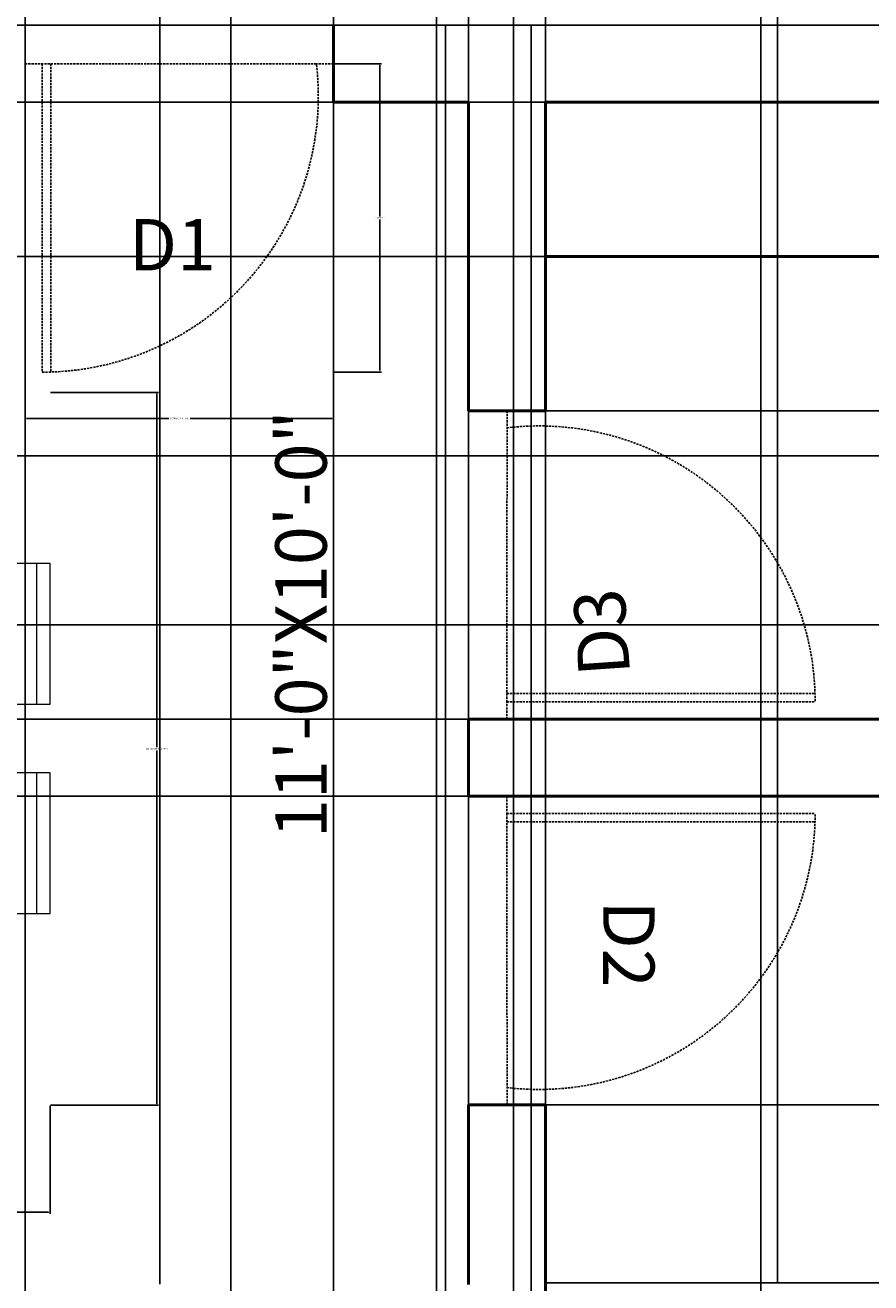
# Model space of a CAD drawing. Units: inches. Extents: x 3 to 576, y -689 to 51.
# Tile 10 of 21: x 336 to 435, y -506 to -359. Entities that reach past the tile are written whole.
import ezdxf

# ---------------------------------------------------------------- set-up
doc = ezdxf.new("R2010")
doc.units = ezdxf.units.IN
doc.header["$MEASUREMENT"] = 0
doc.linetypes.add('DASHED2', pattern=[0.375, 0.25, -0.125])
for name, color, linetype, lineweight in [('A-ANNO-DIMS', 2, 'Continuous', 18), ('A-ANNO-TEXT', 3, 'Continuous', 18), ('A-AREA-IDEN', 7, 'Continuous', 18), ('A-DOOR', 4, 'DASHED2', 25), ('A-FURN', 8, 'Continuous', 18), ('A-WALL', 7, 'Continuous', 50)]:
    doc.layers.add(name, color=color, linetype=linetype, lineweight=lineweight)
doc.styles.get("Standard").update_dxf_attribs({"font": 'arial.ttf'})
doc.dimstyles.get("Standard").update_dxf_attribs({"dimtxt": 0.18, "dimasz": 0.18, "dimexe": 0.18, "dimexo": 0.0625, "dimgap": 0.09, "dimtad": 0, "dimtih": 1, "dimtoh": 1, "dimdec": 0, "dimzin": 0, "dimdsep": 46, "dimlunit": 3, "dimtxsty": 'Standard', "dimcen": 0.09, "dimadec": 0, "dimazin": 0, "dimtfac": 1, "dimtdec": 0, "dimtofl": 0, "dimtmove": 0, "dimatfit": 3, "dimfxl": 1, "dimtolj": 1, "dimtzin": 0, "dimarcsym": 0})

# ---------------------------------------------------------------- blocks, each defined once
blk = doc.blocks.new('DINING-SET-6')
for p, q in [((35.44, 83.21), (19.03, 83.21)), ((19.03, 83.21), (19.03, 74.43)), ((35.44, 74.43), (35.44, 83.21)), ((19.03, 81.61), (35.44, 81.61)), ((37.96, 74.43), (16.08, 74.43)), ((16.08, 72.6), (37.96, 72.6)), ((8.79, 67.13), (8.79, 16.08)), ((10.61, 16.08), (10.61, 67.13)), ((20.49, 66.46), (21.48, 64.87)), ((43.43, 67.13), (43.43, 16.08)), ((45.25, 16.08), (45.25, 67.13)), ((21.9, 63.9), (21.31, 65.43)), ((22.64, 64.98), (21.31, 65.43)), ((21.48, 64.87), (23.07, 63.29)), ((21.9, 63.9), (22.63, 64.98)), ((0, 46.82), (0, 63.23)), ((0, 63.23), (8.79, 63.23)), ((1.6, 63.23), (1.6, 46.82)), ((12.38, 64.08), (12.77, 63.09)), ((23.07, 63.29), (24.85, 62.49)), ((54.04, 63.23), (45.25, 63.23)), ((52.44, 63.23), (52.44, 46.82)), ((54.04, 46.82), (54.04, 63.23)), ((12.77, 63.09), (14.75, 59.12)), ((24.85, 62.49), (25.84, 62.3)), ((25.84, 62.3), (26.44, 61.7)), ((26.44, 61.7), (27.43, 60.91)), ((29.06, 62.49), (27.69, 62.24)), ((28.94, 61.18), (27.69, 62.24)), ((28.94, 61.18), (29.06, 62.49)), ((27.43, 60.91), (28.22, 59.52)), ((12.6, 59.46), (11.23, 59.2)), ((12.49, 58.15), (11.23, 59.2)), ((12.49, 58.15), (12.6, 59.46)), ((14.75, 59.12), (17.52, 55.75)), ((28.22, 59.52), (29.6, 56.55)), ((38.5, 59.66), (37.18, 60.1)), ((37.77, 58.57), (37.18, 60.1)), ((37.77, 58.57), (38.5, 59.66)), ((26.06, 56.77), (23.98, 56.52)), ((25.76, 54.82), (23.98, 56.52)), ((25.76, 54.82), (26.06, 56.77)), ((29.6, 56.55), (30.2, 54.36)), ((30, 56.15), (30.79, 55.36)), ((17.52, 55.75), (18.51, 53.57)), ((30.2, 54.36), (31.39, 52.78)), ((30.79, 55.36), (32.18, 53.97)), ((18.51, 53.57), (18.51, 49.01)), ((32.18, 53.97), (33.96, 53.37)), ((33.96, 53.37), (34.36, 53.18)), ((34.36, 53.18), (35.35, 49.61)), ((13.09, 50.84), (12.5, 52.37)), ((13.83, 51.93), (12.5, 52.37)), ((13.09, 50.84), (13.83, 51.92)), ((31.39, 52.78), (32.77, 51.19)), ((19.11, 51.19), (19.11, 50)), ((19.11, 50), (19.5, 47.82)), ((32.77, 51.19), (33.76, 50.4)), ((33.76, 50.4), (34.75, 46.83)), ((41.09, 49.61), (41.49, 50)), ((18.51, 49.01), (17.52, 46.63)), ((35.35, 49.61), (36.73, 48.22)), ((39.5, 47.23), (41.09, 49.61)), ((43.43, 49.7), (42.77, 49.58)), ((43.43, 49.03), (42.77, 49.58)), ((19.5, 47.82), (19.5, 36.32)), ((28.96, 45.51), (28.37, 47.05)), ((29.69, 46.6), (28.37, 47.05)), ((36.73, 48.22), (37.92, 47.62)), ((37.92, 47.62), (38.71, 47.62)), ((38.71, 47.62), (39.5, 47.23)), ((8.79, 46.82), (0, 46.82)), ((17.52, 46.63), (17.92, 44.25)), ((27.69, 46.8), (26.31, 46.55)), ((27.57, 45.49), (26.31, 46.55)), ((27.57, 45.49), (27.68, 46.8)), ((28.96, 45.51), (29.69, 46.6)), ((34.75, 46.83), (35.15, 44.25)), ((45.25, 46.82), (54.04, 46.82)), ((17.92, 44.25), (18.12, 43.46)), ((19.5, 44.06), (20.09, 43.66)), ((35.15, 44.25), (35.54, 43.06)), ((11.23, 43.76), (10.61, 43.65)), ((11.11, 42.46), (10.61, 42.88)), ((11.11, 42.46), (11.23, 43.76)), ((20.09, 43.66), (21.08, 43.07)), ((21.08, 43.07), (21.68, 42.27)), ((35.54, 43.06), (35.15, 41.68)), ((21.68, 42.27), (22.67, 41.88)), ((22.67, 41.88), (23.46, 41.68)), ((23.46, 41.68), (23.85, 41.68)), ((23.85, 41.68), (24.45, 41.48)), ((35.15, 41.68), (36.14, 40.29)), ((36.14, 40.29), (36.73, 37.12)), ((0, 22.39), (0, 38.8)), ((0, 38.8), (8.79, 38.8)), ((1.6, 38.8), (1.6, 22.39)), ((54.04, 38.8), (45.25, 38.8)), ((52.44, 38.8), (52.44, 22.39)), ((54.04, 22.39), (54.04, 38.8)), ((19.5, 36.32), (19.9, 35.93)), ((19.9, 35.93), (23.27, 33.35)), ((20.15, 32.45), (19.56, 33.99)), ((20.88, 33.54), (19.56, 33.99)), ((42.77, 34.14), (41.4, 33.89)), ((42.65, 32.83), (41.4, 33.89)), ((42.65, 32.83), (42.77, 34.14)), ((20.15, 32.45), (20.88, 33.54)), ((22.44, 33.42), (20.36, 33.17)), ((22.14, 31.47), (20.36, 33.17)), ((22.14, 31.47), (22.44, 33.42)), ((23.27, 33.35), (26.24, 31.57)), ((23.86, 32.95), (25.64, 32.95)), ((25.64, 32.95), (27.03, 32.16)), ((26.31, 31.11), (24.94, 30.85)), ((26.2, 29.8), (24.94, 30.85)), ((26.24, 31.57), (25.84, 28.59)), ((26.2, 29.8), (26.31, 31.11)), ((27.03, 32.16), (27.82, 31.37)), ((27.82, 31.37), (28.81, 30.57)), ((25.84, 28.59), (25.84, 28)), ((36.01, 27.13), (35.43, 28.66)), ((36.75, 28.22), (35.43, 28.66)), ((36.01, 27.13), (36.75, 28.22)), ((40.69, 28), (38.9, 24.23)), ((38.9, 24.23), (38.9, 23.44)), ((8.79, 22.39), (0, 22.39)), ((38.9, 23.44), (39.3, 22.45)), ((39.3, 22.45), (38.9, 20.86)), ((45.25, 22.39), (54.04, 22.39)), ((11.34, 19.39), (10.75, 20.93)), ((12.07, 20.48), (10.75, 20.93)), ((38.9, 20.86), (37.72, 19.87)), ((11.34, 19.39), (12.07, 20.48)), ((30.99, 19.67), (29.8, 20.27)), ((31.78, 16.89), (30.99, 19.67)), ((37.72, 19.87), (37.52, 18.09)), ((37.52, 18.09), (36.92, 16.1)), ((41.28, 17.14), (40.02, 18.2)), ((41.4, 18.45), (40.03, 18.2)), ((41.28, 17.14), (41.4, 18.45)), ((32.18, 16.5), (31.78, 16.89)), ((32.57, 12.93), (32.18, 16.5)), ((24.94, 15.41), (23.57, 15.16)), ((24.82, 14.11), (23.57, 15.16)), ((24.82, 14.11), (24.94, 15.41)), ((27.21, 14.07), (26.62, 15.6)), ((27.94, 15.16), (26.62, 15.6)), ((27.21, 14.07), (27.94, 15.16)), ((36.13, 15.11), (35.74, 14.52)), ((36.92, 16.1), (36.13, 15.11)), ((32.57, 12.53), (32.57, 12.93)), ((35.15, 11.94), (32.57, 12.53)), ((36.14, 11.15), (35.15, 11.94)), ((42.34, 12.8), (41.67, 12.72)), ((42.01, 12.4), (41.67, 12.72)), ((37.96, 10.61), (16.08, 10.61)), ((37.13, 10.75), (36.14, 11.15)), ((16.08, 8.79), (37.96, 8.79)), ((19.03, 8.79), (19.03, 0)), ((35.44, 0), (35.44, 8.79)), ((35.44, 1.6), (19.03, 1.6)), ((19.03, 0), (35.44, 0))]:
    blk.add_line(p, q)
for centre, radius, start, end in [((16.08, 67.13), 7.29, 90, 180), ((37.96, 67.13), 7.29, 0, 90), ((16.08, 67.13), 5.47, 90, 180), ((37.96, 67.13), 5.47, 0, 90), ((16.08, 16.08), 7.29, 180, 270), ((16.08, 16.08), 5.47, 180, 270), ((37.96, 16.08), 5.47, 270, 0), ((37.96, 16.08), 7.29, 270, 0)]:
    blk.add_arc(centre, radius, start, end)
blk = doc.blocks.new('DOOR-SWING-900')
for p, q in [((35.95, 36), (35.95, 34)), ((36, 2), (35.95, 34)), ((36, 2), (0, 2)), ((36, 0), (36, 2))]:
    blk.add_line(p, q)
blk.add_arc((32.22, 2), 32.22, 83.347, 180)
blk = doc.blocks.new('DOOR-900')
for p, q in [((34, 36), (0, 36)), ((2, 36), (2, 0)), ((36, 36), (34, 36))]:
    blk.add_line(p, q)
blk.add_arc((2, 32.22), 32.22, 270, 6.7329)
blk = doc.blocks.new('*D21')
at = {"layer": 'A-ANNO-DIMS', "color": 0, "lineweight": -2, "transparency": 16777216}
for p, q in [((336.29, -399.87), (336.29, -405.39)), ((372.29, -399.87), (372.29, -405.39)), ((336.47, -405.21), (353.05, -405.21)), ((372.11, -405.21), (355.54, -405.21))]:
    blk.add_line(p, q, dxfattribs=at)
at = {"layer": 'A-ANNO-DIMS', "color": 0, "transparency": 16777216}
for points in [[(336.47, -405.18), (336.47, -405.24), (336.29, -405.21)], [(372.11, -405.18), (372.11, -405.24), (372.29, -405.21)]]:
    blk.add_solid(points, dxfattribs=at)
at = {"layer": 'Defpoints', "color": 0, "transparency": 16777216}
for p in [(336.29, -399.81), (372.29, -399.81), (372.29, -405.21)]:
    blk.add_point(p, dxfattribs=at)
at = {"layer": 'A-ANNO-DIMS', "color": 0, "transparency": 16777216, "insert": (354.29, -405.21), "char_height": 0.18, "attachment_point": 5}
blk.add_mtext('\\A1;DOOR D1 3\'-0" TYP.', dxfattribs=at)
blk = doc.blocks.new('*D22')
at = {"layer": 'A-ANNO-DIMS', "color": 0, "lineweight": -2, "transparency": 16777216}
for p, q in [((372.36, -363.81), (377.87, -363.81)), ((377.69, -363.99), (377.69, -381.63)), ((377.69, -399.63), (377.69, -381.99)), ((372.36, -399.81), (377.87, -399.81))]:
    blk.add_line(p, q, dxfattribs=at)
at = {"layer": 'A-ANNO-DIMS', "color": 0, "transparency": 16777216}
for points in [[(377.66, -363.99), (377.72, -363.99), (377.69, -363.81)], [(377.66, -399.63), (377.72, -399.63), (377.69, -399.81)]]:
    blk.add_solid(points, dxfattribs=at)
at = {"layer": 'Defpoints', "color": 0, "transparency": 16777216}
for p in [(372.29, -363.81), (377.69, -363.81), (372.29, -399.81)]:
    blk.add_point(p, dxfattribs=at)
at = {"layer": 'A-ANNO-DIMS', "color": 0, "transparency": 16777216, "insert": (377.69, -381.81), "char_height": 0.18, "attachment_point": 5}
blk.add_mtext('\\A1;3\'-0" TYP.', dxfattribs=at)
blk = doc.blocks.new('*D33')
at = {"layer": 'A-ANNO-DIMS', "color": 0, "lineweight": -2, "transparency": 16777216}
for p, q in [((339.26, -402.17), (351.86, -402.17)), ((351.68, -402.35), (351.68, -443.59)), ((351.68, -485.2), (351.68, -443.96)), ((339.26, -485.38), (351.86, -485.38))]:
    blk.add_line(p, q, dxfattribs=at)
at = {"layer": 'A-ANNO-DIMS', "color": 0, "transparency": 16777216}
for points in [[(351.65, -402.35), (351.71, -402.35), (351.68, -402.17)], [(351.65, -485.2), (351.71, -485.2), (351.68, -485.38)]]:
    blk.add_solid(points, dxfattribs=at)
at = {"layer": 'Defpoints', "color": 0, "transparency": 16777216}
for p in [(339.2, -402.17), (351.68, -402.17), (339.2, -485.38)]:
    blk.add_point(p, dxfattribs=at)
at = {"layer": 'A-ANNO-DIMS', "color": 0, "transparency": 16777216, "insert": (351.68, -443.78), "char_height": 0.18, "attachment_point": 5}
blk.add_mtext('\\A1;DINING SET 6\'-11" TYP.', dxfattribs=at)
blk = doc.blocks.new('*D34')
at = {"layer": 'A-ANNO-DIMS', "color": 0, "lineweight": -2, "transparency": 16777216}
for p, q in [((285.16, -485.45), (285.16, -498.05)), ((339.2, -485.45), (339.2, -498.05)), ((285.34, -497.87), (311.54, -497.87)), ((339.02, -497.87), (312.82, -497.87))]:
    blk.add_line(p, q, dxfattribs=at)
at = {"layer": 'A-ANNO-DIMS', "color": 0, "transparency": 16777216}
for points in [[(285.34, -497.84), (285.34, -497.9), (285.16, -497.87)], [(339.02, -497.84), (339.02, -497.9), (339.2, -497.87)]]:
    blk.add_solid(points, dxfattribs=at)
at = {"layer": 'Defpoints', "color": 0, "transparency": 16777216}
for p in [(285.16, -485.38), (339.2, -485.38), (339.2, -497.87)]:
    blk.add_point(p, dxfattribs=at)
at = {"layer": 'A-ANNO-DIMS', "color": 0, "transparency": 16777216, "insert": (312.18, -497.87), "char_height": 0.18, "attachment_point": 5}
blk.add_mtext('\\A1;4\'-6" TYP.', dxfattribs=at)
blk = doc.blocks.new('*D69')
at = {"layer": 'A-ANNO-DIMS', "color": 0, "lineweight": -2, "transparency": 16777216}
for p, q in [((531.23, -263.31), (2.66, -263.31)), ((2.84, -263.49), (2.84, -311.13)), ((2.84, -359.13), (2.84, -311.49)), ((531.23, -359.31), (2.66, -359.31))]:
    blk.add_line(p, q, dxfattribs=at)
at = {"layer": 'A-ANNO-DIMS', "color": 0, "transparency": 16777216}
for points in [[(2.81, -263.49), (2.87, -263.49), (2.84, -263.31)], [(2.81, -359.13), (2.87, -359.13), (2.84, -359.31)]]:
    blk.add_solid(points, dxfattribs=at)
at = {"layer": 'Defpoints', "color": 0, "transparency": 16777216}
for p in [(531.29, -263.31), (2.84, -359.31), (531.29, -359.31)]:
    blk.add_point(p, dxfattribs=at)
at = {"layer": 'A-ANNO-DIMS', "color": 0, "transparency": 16777216, "insert": (2.84, -311.31), "char_height": 0.18, "attachment_point": 5}
blk.add_mtext('\\A1;8\'-0"', dxfattribs=at)
blk = doc.blocks.new('*D70')
at = {"layer": 'A-ANNO-DIMS', "color": 0, "lineweight": -2, "transparency": 16777216}
for p, q in [((531.23, -359.31), (2.66, -359.31)), ((2.84, -359.49), (2.84, -363.63)), ((2.84, -368.13), (2.84, -363.99)), ((531.23, -368.31), (2.66, -368.31))]:
    blk.add_line(p, q, dxfattribs=at)
at = {"layer": 'A-ANNO-DIMS', "color": 0, "transparency": 16777216}
for points in [[(2.81, -359.49), (2.87, -359.49), (2.84, -359.31)], [(2.81, -368.13), (2.87, -368.13), (2.84, -368.31)]]:
    blk.add_solid(points, dxfattribs=at)
at = {"layer": 'Defpoints', "color": 0, "transparency": 16777216}
for p in [(531.29, -359.31), (2.84, -368.31), (531.29, -368.31)]:
    blk.add_point(p, dxfattribs=at)
at = {"layer": 'A-ANNO-DIMS', "color": 0, "transparency": 16777216, "insert": (2.84, -363.81), "char_height": 0.18, "attachment_point": 5}
blk.add_mtext('\\A1;0\'-9"', dxfattribs=at)
blk = doc.blocks.new('*D71')
at = {"layer": 'A-ANNO-DIMS', "color": 0, "lineweight": -2, "transparency": 16777216}
for p, q in [((531.23, -368.31), (2.66, -368.31)), ((2.84, -368.49), (2.84, -404.13)), ((2.84, -440.13), (2.84, -404.49)), ((531.23, -440.31), (2.66, -440.31))]:
    blk.add_line(p, q, dxfattribs=at)
at = {"layer": 'A-ANNO-DIMS', "color": 0, "transparency": 16777216}
for points in [[(2.81, -368.49), (2.87, -368.49), (2.84, -368.31)], [(2.81, -440.13), (2.87, -440.13), (2.84, -440.31)]]:
    blk.add_solid(points, dxfattribs=at)
at = {"layer": 'Defpoints', "color": 0, "transparency": 16777216}
for p in [(531.29, -368.31), (2.84, -440.31), (531.29, -440.31)]:
    blk.add_point(p, dxfattribs=at)
at = {"layer": 'A-ANNO-DIMS', "color": 0, "transparency": 16777216, "insert": (2.84, -404.31), "char_height": 0.18, "attachment_point": 5}
blk.add_mtext('\\A1;6\'-0"', dxfattribs=at)
blk = doc.blocks.new('*D72')
at = {"layer": 'A-ANNO-DIMS', "color": 0, "lineweight": -2, "transparency": 16777216}
for p, q in [((531.23, -440.31), (2.66, -440.31)), ((2.84, -440.49), (2.84, -444.63)), ((2.84, -449.13), (2.84, -444.99)), ((531.23, -449.31), (2.66, -449.31))]:
    blk.add_line(p, q, dxfattribs=at)
at = {"layer": 'A-ANNO-DIMS', "color": 0, "transparency": 16777216}
for points in [[(2.81, -440.49), (2.87, -440.49), (2.84, -440.31)], [(2.81, -449.13), (2.87, -449.13), (2.84, -449.31)]]:
    blk.add_solid(points, dxfattribs=at)
at = {"layer": 'Defpoints', "color": 0, "transparency": 16777216}
for p in [(531.29, -440.31), (2.84, -449.31), (531.29, -449.31)]:
    blk.add_point(p, dxfattribs=at)
at = {"layer": 'A-ANNO-DIMS', "color": 0, "transparency": 16777216, "insert": (2.84, -444.81), "char_height": 0.18, "attachment_point": 5}
blk.add_mtext('\\A1;0\'-9"', dxfattribs=at)
blk = doc.blocks.new('*D73')
at = {"layer": 'A-ANNO-DIMS', "color": 0, "lineweight": -2, "transparency": 16777216}
for p, q in [((531.23, -449.31), (2.66, -449.31)), ((2.84, -449.49), (2.84, -518.13)), ((2.84, -587.13), (2.84, -518.49)), ((531.23, -587.31), (2.66, -587.31))]:
    blk.add_line(p, q, dxfattribs=at)
at = {"layer": 'A-ANNO-DIMS', "color": 0, "transparency": 16777216}
for points in [[(2.81, -449.49), (2.87, -449.49), (2.84, -449.31)], [(2.81, -587.13), (2.87, -587.13), (2.84, -587.31)]]:
    blk.add_solid(points, dxfattribs=at)
at = {"layer": 'Defpoints', "color": 0, "transparency": 16777216}
for p in [(531.29, -449.31), (2.84, -587.31), (531.29, -587.31)]:
    blk.add_point(p, dxfattribs=at)
at = {"layer": 'A-ANNO-DIMS', "color": 0, "transparency": 16777216, "insert": (2.84, -518.31), "char_height": 0.18, "attachment_point": 5}
blk.add_mtext('\\A1;11\'-6"', dxfattribs=at)
blk = doc.blocks.new('*D76')
at = {"layer": 'A-ANNO-DIMS', "color": 0, "lineweight": -2, "transparency": 16777216}
for p, q in [((372.29, -263.37), (372.29, -688.94)), ((336.29, -296.37), (336.29, -688.94)), ((336.47, -688.76), (353.96, -688.76)), ((372.11, -688.76), (354.62, -688.76))]:
    blk.add_line(p, q, dxfattribs=at)
at = {"layer": 'A-ANNO-DIMS', "color": 0, "transparency": 16777216}
for points in [[(336.47, -688.73), (336.47, -688.79), (336.29, -688.76)], [(372.11, -688.73), (372.11, -688.79), (372.29, -688.76)]]:
    blk.add_solid(points, dxfattribs=at)
at = {"layer": 'Defpoints', "color": 0, "transparency": 16777216}
for p in [(372.29, -263.31), (336.29, -296.31), (372.29, -688.76)]:
    blk.add_point(p, dxfattribs=at)
at = {"layer": 'A-ANNO-DIMS', "color": 0, "transparency": 16777216, "insert": (354.29, -688.76), "char_height": 0.18, "attachment_point": 5}
blk.add_mtext('\\A1;3\'-0"', dxfattribs=at)
blk = doc.blocks.new('*D77')
at = {"layer": 'A-ANNO-DIMS', "color": 0, "lineweight": -2, "transparency": 16777216}
for p, q in [((372.29, -263.37), (372.29, -688.94)), ((531.29, -263.37), (531.29, -688.94)), ((372.47, -688.76), (451.4, -688.76)), ((531.11, -688.76), (452.18, -688.76))]:
    blk.add_line(p, q, dxfattribs=at)
at = {"layer": 'A-ANNO-DIMS', "color": 0, "transparency": 16777216}
for points in [[(372.47, -688.73), (372.47, -688.79), (372.29, -688.76)], [(531.11, -688.73), (531.11, -688.79), (531.29, -688.76)]]:
    blk.add_solid(points, dxfattribs=at)
at = {"layer": 'Defpoints', "color": 0, "transparency": 16777216}
for p in [(372.29, -263.31), (531.29, -263.31), (531.29, -688.76)]:
    blk.add_point(p, dxfattribs=at)
at = {"layer": 'A-ANNO-DIMS', "color": 0, "transparency": 16777216, "insert": (451.79, -688.76), "char_height": 0.18, "attachment_point": 5}
blk.add_mtext('\\A1;13\'-3"', dxfattribs=at)
blk = doc.blocks.new('*D80')
at = {"layer": 'A-ANNO-DIMS', "color": 0, "lineweight": -2, "transparency": 16777216}
for p, q in [((372.29, -359.37), (372.29, -688.94)), ((385.37, -359.37), (385.37, -688.94)), ((372.47, -688.76), (378.51, -688.76)), ((385.19, -688.76), (379.15, -688.76))]:
    blk.add_line(p, q, dxfattribs=at)
at = {"layer": 'A-ANNO-DIMS', "color": 0, "transparency": 16777216}
for points in [[(372.47, -688.73), (372.47, -688.79), (372.29, -688.76)], [(385.19, -688.73), (385.19, -688.79), (385.37, -688.76)]]:
    blk.add_solid(points, dxfattribs=at)
at = {"layer": 'Defpoints', "color": 0, "transparency": 16777216}
for p in [(372.29, -359.31), (385.37, -359.31), (385.37, -688.76)]:
    blk.add_point(p, dxfattribs=at)
at = {"layer": 'A-ANNO-DIMS', "color": 0, "transparency": 16777216, "insert": (378.83, -688.76), "char_height": 0.18, "attachment_point": 5}
blk.add_mtext('\\A1;1\'-1"', dxfattribs=at)
blk = doc.blocks.new('*D81')
at = {"layer": 'A-ANNO-DIMS', "color": 0, "lineweight": -2, "transparency": 16777216}
for p, q in [((385.37, -359.37), (385.37, -688.94)), ((395.37, -359.37), (395.37, -688.94)), ((385.55, -688.76), (389.97, -688.76)), ((395.19, -688.76), (390.76, -688.76))]:
    blk.add_line(p, q, dxfattribs=at)
at = {"layer": 'A-ANNO-DIMS', "color": 0, "transparency": 16777216}
for points in [[(385.55, -688.73), (385.55, -688.79), (385.37, -688.76)], [(395.19, -688.73), (395.19, -688.79), (395.37, -688.76)]]:
    blk.add_solid(points, dxfattribs=at)
at = {"layer": 'Defpoints', "color": 0, "transparency": 16777216}
for p in [(385.37, -359.31), (395.37, -359.31), (395.37, -688.76)]:
    blk.add_point(p, dxfattribs=at)
at = {"layer": 'A-ANNO-DIMS', "color": 0, "transparency": 16777216, "insert": (390.37, -688.76), "char_height": 0.18, "attachment_point": 5}
blk.add_mtext('\\A1;0\'-10"', dxfattribs=at)
blk = doc.blocks.new('*D82')
at = {"layer": 'A-ANNO-DIMS', "color": 0, "lineweight": -2, "transparency": 16777216}
for p, q in [((395.37, -359.37), (395.37, -688.94)), ((475.37, -359.37), (475.37, -688.94)), ((395.55, -688.76), (435.04, -688.76)), ((475.19, -688.76), (435.7, -688.76))]:
    blk.add_line(p, q, dxfattribs=at)
at = {"layer": 'A-ANNO-DIMS', "color": 0, "transparency": 16777216}
for points in [[(395.55, -688.73), (395.55, -688.79), (395.37, -688.76)], [(475.19, -688.73), (475.19, -688.79), (475.37, -688.76)]]:
    blk.add_solid(points, dxfattribs=at)
at = {"layer": 'Defpoints', "color": 0, "transparency": 16777216}
for p in [(395.37, -359.31), (475.37, -359.31), (475.37, -688.76)]:
    blk.add_point(p, dxfattribs=at)
at = {"layer": 'A-ANNO-DIMS', "color": 0, "transparency": 16777216, "insert": (435.37, -688.76), "char_height": 0.18, "attachment_point": 5}
blk.add_mtext('\\A1;6\'-8"', dxfattribs=at)
blk = doc.blocks.new('*D85')
at = {"layer": 'A-ANNO-DIMS', "color": 0, "lineweight": -2, "transparency": 16777216}
for p, q in [((385.3, -313.31), (2.66, -313.31)), ((2.84, -313.49), (2.84, -336.13)), ((2.84, -359.13), (2.84, -336.49)), ((385.3, -359.31), (2.66, -359.31))]:
    blk.add_line(p, q, dxfattribs=at)
at = {"layer": 'A-ANNO-DIMS', "color": 0, "transparency": 16777216}
for points in [[(2.81, -313.49), (2.87, -313.49), (2.84, -313.31)], [(2.81, -359.13), (2.87, -359.13), (2.84, -359.31)]]:
    blk.add_solid(points, dxfattribs=at)
at = {"layer": 'Defpoints', "color": 0, "transparency": 16777216}
for p in [(385.37, -313.31), (2.84, -359.31), (385.37, -359.31)]:
    blk.add_point(p, dxfattribs=at)
at = {"layer": 'A-ANNO-DIMS', "color": 0, "transparency": 16777216, "insert": (2.84, -336.31), "char_height": 0.18, "attachment_point": 5}
blk.add_mtext('\\A1;3\'-10"', dxfattribs=at)
blk = doc.blocks.new('*D91')
at = {"layer": 'A-ANNO-DIMS', "color": 0, "lineweight": -2, "transparency": 16777216}
for p, q in [((181.1, -386.31), (575.92, -386.31)), ((575.74, -386.49), (575.74, -397.75)), ((575.74, -409.38), (575.74, -398.11)), ((181.1, -409.56), (575.92, -409.56))]:
    blk.add_line(p, q, dxfattribs=at)
at = {"layer": 'A-ANNO-DIMS', "color": 0, "transparency": 16777216}
for points in [[(575.71, -386.49), (575.77, -386.49), (575.74, -386.31)], [(575.71, -409.38), (575.77, -409.38), (575.74, -409.56)]]:
    blk.add_solid(points, dxfattribs=at)
at = {"layer": 'Defpoints', "color": 0, "transparency": 16777216}
for p in [(181.04, -386.31), (181.04, -409.56), (575.74, -409.56)]:
    blk.add_point(p, dxfattribs=at)
at = {"layer": 'A-ANNO-DIMS', "color": 0, "transparency": 16777216, "insert": (575.74, -397.93), "char_height": 0.18, "attachment_point": 5}
blk.add_mtext('\\A1;1\'-11"', dxfattribs=at)
blk = doc.blocks.new('*D94')
at = {"layer": 'A-ANNO-DIMS', "color": 0, "lineweight": -2, "transparency": 16777216}
for p, q in [((393.29, -136.9), (393.29, -688.94)), ((422.14, -136.9), (422.14, -688.94)), ((393.47, -688.76), (407.39, -688.76)), ((421.96, -688.76), (408.05, -688.76))]:
    blk.add_line(p, q, dxfattribs=at)
at = {"layer": 'A-ANNO-DIMS', "color": 0, "transparency": 16777216}
for points in [[(393.47, -688.73), (393.47, -688.79), (393.29, -688.76)], [(421.96, -688.73), (421.96, -688.79), (422.14, -688.76)]]:
    blk.add_solid(points, dxfattribs=at)
at = {"layer": 'Defpoints', "color": 0, "transparency": 16777216}
for p in [(393.29, -136.84), (422.14, -136.84), (422.14, -688.76)]:
    blk.add_point(p, dxfattribs=at)
at = {"layer": 'A-ANNO-DIMS', "color": 0, "transparency": 16777216, "insert": (407.72, -688.76), "char_height": 0.18, "attachment_point": 5}
blk.add_mtext('\\A1;2\'-5"', dxfattribs=at)
blk = doc.blocks.new('*D96')
at = {"layer": 'A-ANNO-DIMS', "color": 0, "lineweight": -2, "transparency": 16777216}
for p, q in [((397.02, -506.04), (397.02, 51.32)), ((397.2, 51.14), (410.22, 51.14)), ((423.91, 51.14), (410.89, 51.14)), ((424.09, -506.04), (424.09, 51.32))]:
    blk.add_line(p, q, dxfattribs=at)
at = {"layer": 'A-ANNO-DIMS', "color": 0, "transparency": 16777216}
for points in [[(397.2, 51.17), (397.2, 51.11), (397.02, 51.14)], [(423.91, 51.17), (423.91, 51.11), (424.09, 51.14)]]:
    blk.add_solid(points, dxfattribs=at)
at = {"layer": 'Defpoints', "color": 0, "transparency": 16777216}
for p in [(424.09, 51.14), (397.02, -506.1), (424.09, -506.1)]:
    blk.add_point(p, dxfattribs=at)
at = {"layer": 'A-ANNO-DIMS', "color": 0, "transparency": 16777216, "insert": (410.56, 51.14), "char_height": 0.18, "attachment_point": 5}
blk.add_mtext('\\A1;2\'-3"', dxfattribs=at)
blk = doc.blocks.new('*D97')
at = {"layer": 'A-ANNO-DIMS', "color": 0, "lineweight": -2, "transparency": 16777216}
for p, q in [((424.15, -506.1), (575.92, -506.1)), ((575.74, -506.28), (575.74, -546.52)), ((575.74, -587.13), (575.74, -546.89)), ((424.15, -587.31), (575.92, -587.31))]:
    blk.add_line(p, q, dxfattribs=at)
at = {"layer": 'A-ANNO-DIMS', "color": 0, "transparency": 16777216}
for points in [[(575.71, -506.28), (575.77, -506.28), (575.74, -506.1)], [(575.71, -587.13), (575.77, -587.13), (575.74, -587.31)]]:
    blk.add_solid(points, dxfattribs=at)
at = {"layer": 'Defpoints', "color": 0, "transparency": 16777216}
for p in [(424.09, -506.1), (424.09, -587.31), (575.74, -587.31)]:
    blk.add_point(p, dxfattribs=at)
at = {"layer": 'A-ANNO-DIMS', "color": 0, "transparency": 16777216, "insert": (575.74, -546.71), "char_height": 0.18, "attachment_point": 5}
blk.add_mtext('\\A1;6\'-9"', dxfattribs=at)
blk = doc.blocks.new('*D106')
at = {"layer": 'A-ANNO-DIMS', "color": 0, "lineweight": -2, "transparency": 16777216}
for p, q in [((111.36, -386.31), (575.92, -386.31)), ((575.74, -386.49), (575.74, -407.63)), ((575.74, -429.13), (575.74, -407.99)), ((111.36, -429.31), (575.92, -429.31))]:
    blk.add_line(p, q, dxfattribs=at)
at = {"layer": 'A-ANNO-DIMS', "color": 0, "transparency": 16777216}
for points in [[(575.71, -386.49), (575.77, -386.49), (575.74, -386.31)], [(575.71, -429.13), (575.77, -429.13), (575.74, -429.31)]]:
    blk.add_solid(points, dxfattribs=at)
at = {"layer": 'Defpoints', "color": 0, "transparency": 16777216}
for p in [(111.29, -386.31), (111.29, -429.31), (575.74, -429.31)]:
    blk.add_point(p, dxfattribs=at)
at = {"layer": 'A-ANNO-DIMS', "color": 0, "transparency": 16777216, "insert": (575.74, -407.81), "char_height": 0.18, "attachment_point": 5}
blk.add_mtext('\\A1;3\'-7"', dxfattribs=at)
blk = doc.blocks.new('*D110')
at = {"layer": 'A-ANNO-DIMS', "color": 0, "lineweight": -2, "transparency": 16777216}
for p, q in [((397.08, -368.31), (575.92, -368.31)), ((575.74, -368.49), (575.74, -386.13)), ((575.74, -404.13), (575.74, -386.49)), ((397.08, -404.31), (575.92, -404.31))]:
    blk.add_line(p, q, dxfattribs=at)
at = {"layer": 'A-ANNO-DIMS', "color": 0, "transparency": 16777216}
for points in [[(575.71, -368.49), (575.77, -368.49), (575.74, -368.31)], [(575.71, -404.13), (575.77, -404.13), (575.74, -404.31)]]:
    blk.add_solid(points, dxfattribs=at)
at = {"layer": 'Defpoints', "color": 0, "transparency": 16777216}
for p in [(397.02, -368.31), (397.02, -404.31), (575.74, -404.31)]:
    blk.add_point(p, dxfattribs=at)
at = {"layer": 'A-ANNO-DIMS', "color": 0, "transparency": 16777216, "insert": (575.74, -386.31), "char_height": 0.18, "attachment_point": 5}
blk.add_mtext('\\A1;3\'-0"', dxfattribs=at)
blk = doc.blocks.new('*D111')
at = {"layer": 'A-ANNO-DIMS', "color": 0, "lineweight": -2, "transparency": 16777216}
for p, q in [((397.08, -485.31), (575.92, -485.31)), ((575.74, -485.49), (575.74, -495.52)), ((575.74, -505.92), (575.74, -495.89)), ((397.08, -506.1), (575.92, -506.1))]:
    blk.add_line(p, q, dxfattribs=at)
at = {"layer": 'A-ANNO-DIMS', "color": 0, "transparency": 16777216}
for points in [[(575.71, -485.49), (575.77, -485.49), (575.74, -485.31)], [(575.71, -505.92), (575.77, -505.92), (575.74, -506.1)]]:
    blk.add_solid(points, dxfattribs=at)
at = {"layer": 'Defpoints', "color": 0, "transparency": 16777216}
for p in [(397.02, -485.31), (397.02, -506.1), (575.74, -506.1)]:
    blk.add_point(p, dxfattribs=at)
at = {"layer": 'A-ANNO-DIMS', "color": 0, "transparency": 16777216, "insert": (575.74, -495.71), "char_height": 0.18, "attachment_point": 5}
blk.add_mtext('\\A1;1\'-9"', dxfattribs=at)
blk = doc.blocks.new('*D116')
at = {"layer": 'A-ANNO-DIMS', "color": 0, "lineweight": -2, "transparency": 16777216}
for p, q in [((360.29, -134.37), (360.29, -688.94)), ((384.29, -134.37), (384.29, -688.94)), ((360.47, -688.76), (371.96, -688.76)), ((384.11, -688.76), (372.62, -688.76))]:
    blk.add_line(p, q, dxfattribs=at)
at = {"layer": 'A-ANNO-DIMS', "color": 0, "transparency": 16777216}
for points in [[(360.47, -688.73), (360.47, -688.79), (360.29, -688.76)], [(384.11, -688.73), (384.11, -688.79), (384.29, -688.76)]]:
    blk.add_solid(points, dxfattribs=at)
at = {"layer": 'Defpoints', "color": 0, "transparency": 16777216}
for p in [(360.29, -134.31), (384.29, -134.31), (384.29, -688.76)]:
    blk.add_point(p, dxfattribs=at)
at = {"layer": 'A-ANNO-DIMS', "color": 0, "transparency": 16777216, "insert": (372.29, -688.76), "char_height": 0.18, "attachment_point": 5}
blk.add_mtext('\\A1;2\'-0"', dxfattribs=at)
blk = doc.blocks.new('*D118')
at = {"layer": 'A-ANNO-DIMS', "color": 0, "lineweight": -2, "transparency": 16777216}
for p, q in [((352.02, -506.25), (352.02, 51.32)), ((352.2, 51.14), (369.69, 51.14)), ((387.84, 51.14), (370.35, 51.14)), ((388.02, -506.25), (388.02, 51.32))]:
    blk.add_line(p, q, dxfattribs=at)
at = {"layer": 'A-ANNO-DIMS', "color": 0, "transparency": 16777216}
for points in [[(352.2, 51.17), (352.2, 51.11), (352.02, 51.14)], [(387.84, 51.17), (387.84, 51.11), (388.02, 51.14)]]:
    blk.add_solid(points, dxfattribs=at)
at = {"layer": 'Defpoints', "color": 0, "transparency": 16777216}
for p in [(388.02, 51.14), (352.02, -506.31), (388.02, -506.31)]:
    blk.add_point(p, dxfattribs=at)
at = {"layer": 'A-ANNO-DIMS', "color": 0, "transparency": 16777216, "insert": (370.02, 51.14), "char_height": 0.18, "attachment_point": 5}
blk.add_mtext('\\A1;3\'-0"', dxfattribs=at)
blk = doc.blocks.new('*D125')
at = {"layer": 'A-ANNO-DIMS', "color": 0, "lineweight": -2, "transparency": 16777216}
for p, q in [((531.23, -368.31), (2.66, -368.31)), ((2.84, -368.49), (2.84, -377.13)), ((2.84, -386.13), (2.84, -377.49)), ((512.45, -386.31), (2.66, -386.31))]:
    blk.add_line(p, q, dxfattribs=at)
at = {"layer": 'A-ANNO-DIMS', "color": 0, "transparency": 16777216}
for points in [[(2.81, -368.49), (2.87, -368.49), (2.84, -368.31)], [(2.81, -386.13), (2.87, -386.13), (2.84, -386.31)]]:
    blk.add_solid(points, dxfattribs=at)
at = {"layer": 'Defpoints', "color": 0, "transparency": 16777216}
for p in [(531.29, -368.31), (2.84, -386.31), (512.51, -386.31)]:
    blk.add_point(p, dxfattribs=at)
at = {"layer": 'A-ANNO-DIMS', "color": 0, "transparency": 16777216, "insert": (2.84, -377.31), "char_height": 0.18, "attachment_point": 5}
blk.add_mtext('\\A1;1\'-6"', dxfattribs=at)

msp = doc.modelspace()

# ---------------------------------------------------------------- linework, layer by layer
at = {"layer": 'A-DOOR'}
for p, q in [((339.29, -363.81), (339.29, -399.81)), ((392.52, -437.31), (428.52, -437.31)), ((392.52, -452.31), (428.52, -452.31))]:
    msp.add_line(p, q, dxfattribs=at)
at = {"layer": 'A-WALL'}
for p, q in [((372.29, -368.31), (372.29, -359.31)), ((372.29, -368.31), (388.02, -368.31)), ((388.02, -368.31), (388.02, -404.31)), ((397.02, -368.31), (397.02, -404.31)), ((397.02, -368.31), (531.29, -368.31)), ((397.02, -386.31), (512.51, -386.31)), ((397.02, -404.31), (388.02, -404.31)), ((388.02, -440.31), (531.29, -440.31)), ((388.02, -440.31), (388.02, -449.31)), ((388.02, -449.31), (531.29, -449.31)), ((388.02, -485.31), (397.02, -485.31)), ((388.02, -485.31), (388.02, -506.31)), ((397.02, -485.31), (397.02, -587.31))]:
    msp.add_line(p, q, dxfattribs=at)

# ---------------------------------------------------------------- block references
at = {"layer": 'A-DOOR'}
msp.add_blockref('DOOR-900', (336.29, -399.81), dxfattribs=at)
at = {"layer": 'A-DOOR', "extrusion": (0, 0, -1), "zscale": -1, "rotation": 359.9872034024854}
msp.add_blockref('DOOR-SWING-900', (-428.5, -440.3), dxfattribs=at)
at = {"layer": 'A-DOOR', "rotation": 179.9872034024853}
msp.add_blockref('DOOR-SWING-900', (428.5, -449.32), dxfattribs=at)
at = {"layer": 'A-FURN'}
msp.add_blockref('DINING-SET-6', (285.16, -485.38), dxfattribs=at)

# ---------------------------------------------------------------- texts
at = {"layer": 'A-ANNO-TEXT', "insert": (348.39, -381.94), "char_height": 6, "attachment_point": 1}
msp.add_mtext('D1', dxfattribs=at)
at = {"layer": 'A-ANNO-TEXT', "char_height": 6, "attachment_point": 1}
for s, insert, rotation in [('D3', (400.92, -435.48), 93.9449), ('D2', (409.77, -461.49), 269.7552)]:
    msp.add_mtext(s, dxfattribs=dict(at, insert=insert, rotation=rotation))
at = {"layer": 'A-AREA-IDEN', "insert": (365.49, -454.19), "char_height": 6, "attachment_point": 1, "rotation": 90}
msp.add_mtext('11\'-0"X10\'-0"', dxfattribs=at)

# ---------------------------------------------------------------- dimensions: what is measured, and where the dimension line sits
at = {"layer": 'A-ANNO-DIMS'}
for base, p1, p2, picture, middle in [((388.02, 51.14), (352.02, -506.31), (388.02, -506.31), '*D118', (370.02, 51.14)), ((424.09, 51.14), (397.02, -506.1), (424.09, -506.1), '*D96', (410.56, 51.14)), ((384.29, -688.76), (360.29, -134.31), (384.29, -134.31), '*D116', (372.29, -688.76)), ((422.1383, -688.7597), (393.294, -136.8425), (422.1383, -136.8425), '*D94', (407.7162, -688.7597)), ((372.29, -688.76), (336.29, -296.31), (372.29, -263.31), '*D76', (354.29, -688.76)), ((531.29, -688.76), (372.29, -263.31), (531.29, -263.31), '*D77', (451.79, -688.76)), ((385.37, -688.76), (372.29, -359.31), (385.37, -359.31), '*D80', (378.83, -688.76)), ((395.37, -688.76), (385.37, -359.31), (395.37, -359.31), '*D81', (390.37, -688.76)), ((475.37, -688.76), (395.37, -359.31), (475.37, -359.31), '*D82', (435.37, -688.76))]:
    dim = msp.add_linear_dim(base=base, p1=p1, p2=p2, dimstyle='Standard', override={"dimdec": 1, "dimlfac": 1, "dimrnd": 0, "dimzin": 1, "dimdsep": 46, "dimlunit": 4, "dimfrac": 2}, dxfattribs=at)
    dim.commit()
    dim.dimension.update_dxf_attribs({"geometry": picture, "text_midpoint": middle})
for base, p1, p2, picture, middle in [((2.84, -359.31), (531.29, -263.31), (531.29, -359.31), '*D69', (2.84, -311.31)), ((2.84, -359.31), (385.37, -313.31), (385.37, -359.31), '*D85', (2.84, -336.31)), ((2.84, -368.31), (531.29, -359.31), (531.29, -368.31), '*D70', (2.84, -363.81)), ((2.84, -440.31), (531.29, -368.31), (531.29, -440.31), '*D71', (2.84, -404.31)), ((2.84, -386.31), (531.29, -368.31), (512.51, -386.31), '*D125', (2.84, -377.31)), ((575.74, -404.31), (397.02, -368.31), (397.02, -404.31), '*D110', (575.74, -386.31)), ((575.74, -429.31), (111.29, -386.31), (111.29, -429.31), '*D106', (575.74, -407.81)), ((575.744, -409.5571), (181.036, -386.3097), (181.036, -409.5571), '*D91', (575.744, -397.9334)), ((2.84, -449.31), (531.29, -440.31), (531.29, -449.31), '*D72', (2.84, -444.81)), ((2.84, -587.31), (531.29, -449.31), (531.29, -587.31), '*D73', (2.84, -518.31)), ((575.74, -506.1), (397.02, -485.31), (397.02, -506.1), '*D111', (575.74, -495.71)), ((575.74, -587.31), (424.09, -506.1), (424.09, -587.31), '*D97', (575.74, -546.71))]:
    dim = msp.add_linear_dim(base=base, p1=p1, p2=p2, angle=90, dimstyle='Standard', override={"dimdec": 1, "dimlfac": 1, "dimrnd": 0, "dimzin": 1, "dimdsep": 46, "dimlunit": 4, "dimfrac": 2}, dxfattribs=at)
    dim.commit()
    dim.dimension.update_dxf_attribs({"geometry": picture, "text_midpoint": middle})
for base, p1, p2, text, picture, middle in [((377.69, -363.81), (372.29, -399.81), (372.29, -363.81), '<> TYP.', '*D22', (377.69, -381.81)), ((351.68, -402.17), (339.2, -485.38), (339.2, -402.17), 'DINING SET <> TYP.', '*D33', (351.68, -443.78))]:
    dim = msp.add_linear_dim(base=base, p1=p1, p2=p2, angle=90, text=text, dimstyle='Standard', override={"dimdec": 1, "dimlfac": 1, "dimrnd": 0, "dimzin": 1, "dimdsep": 46, "dimlunit": 4, "dimfrac": 2}, dxfattribs=at)
    dim.commit()
    dim.dimension.update_dxf_attribs({"geometry": picture, "text_midpoint": middle})
for base, p1, p2, text, picture, middle in [((372.29, -405.21), (336.29, -399.81), (372.29, -399.81), 'DOOR D1 <> TYP.', '*D21', (354.29, -405.21)), ((339.2, -497.87), (285.16, -485.38), (339.2, -485.38), '<> TYP.', '*D34', (312.18, -497.87))]:
    dim = msp.add_linear_dim(base=base, p1=p1, p2=p2, text=text, dimstyle='Standard', override={"dimdec": 1, "dimlfac": 1, "dimrnd": 0, "dimzin": 1, "dimdsep": 46, "dimlunit": 4, "dimfrac": 2}, dxfattribs=at)
    dim.commit()
    dim.dimension.update_dxf_attribs({"geometry": picture, "text_midpoint": middle})

doc.saveas('drawing.dxf')
